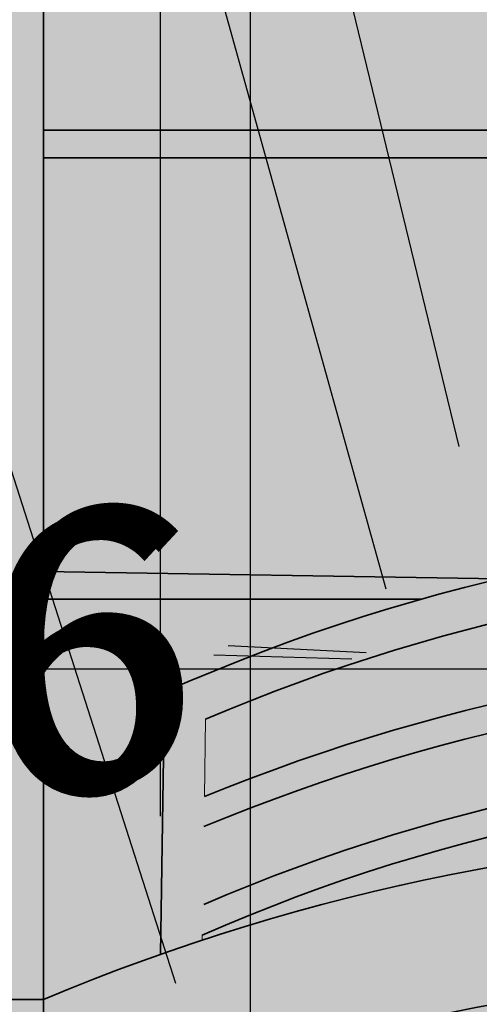
# Model space of a CAD drawing. Units: millimetres. Extents: x 130 to 1021, y 147 to 699.
# Tile 20 of 40: x 366 to 399, y 477 to 548. Entities that reach past the tile are written whole.
import ezdxf

# ---------------------------------------------------------------- set-up
doc = ezdxf.new("R2010")
doc.units = ezdxf.units.MM
doc.header["$MEASUREMENT"] = 0
for name, color, linetype, lineweight in [('A-ANNO-DIMS', 2, 'Continuous', 18), ('A-ELEV', 7, 'Continuous', 35), ('A-ELEV-PATT', 9, 'Continuous', 13), ('A-ELEV-RAIL', 6, 'Continuous', 18)]:
    doc.layers.add(name, color=color, linetype=linetype, lineweight=lineweight)
doc.styles.get("Standard").update_dxf_attribs({"font": 'arial.ttf'})
doc.dimstyles.get("Standard").update_dxf_attribs({"dimtxt": 20, "dimasz": 10, "dimexe": 10, "dimexo": 10, "dimgap": 5, "dimtad": 0, "dimtih": 1, "dimtoh": 1, "dimdec": 0, "dimzin": 0, "dimdsep": 46, "dimtxsty": 'Standard', "dimcen": 5, "dimadec": 0, "dimazin": 0, "dimtfac": 1, "dimtdec": 0, "dimtofl": 0, "dimtmove": 0, "dimatfit": 3, "dimfxl": 1, "dimtolj": 1, "dimtzin": 0, "dimarcsym": 0})

# ---------------------------------------------------------------- blocks, each defined once
blk = doc.blocks.new('*D11')
at = {"layer": 'A-ANNO-DIMS', "color": 0, "lineweight": -2, "transparency": 16777216}
for p, q in [((737.374, 648.699), (737.374, 149.739)), ((299.374, 566.947), (299.374, 149.739)), ((309.374, 159.739), (490.857, 159.739)), ((727.374, 159.739), (545.891, 159.739))]:
    blk.add_line(p, q, dxfattribs=at)
at = {"layer": 'A-ANNO-DIMS', "color": 0, "transparency": 16777216}
for points in [[(309.374, 161.406), (309.374, 158.073), (299.374, 159.739)], [(727.374, 161.406), (727.374, 158.073), (737.374, 159.739)]]:
    blk.add_solid(points, dxfattribs=at)
at = {"layer": 'Defpoints', "color": 0, "transparency": 16777216}
for p in [(737.374, 658.699), (299.374, 576.947), (737.374, 159.739)]:
    blk.add_point(p, dxfattribs=at)
at = {"layer": 'A-ANNO-DIMS', "color": 0, "transparency": 16777216, "insert": (518.374, 159.739), "char_height": 20, "attachment_point": 5}
blk.add_mtext('\\A1;438', dxfattribs=at)
blk = doc.blocks.new('*D12')
at = {"layer": 'A-ANNO-DIMS', "color": 0, "lineweight": -2, "transparency": 16777216}
for p, q in [((477.374, 661.947), (265.074, 661.947)), ((275.074, 651.947), (275.074, 438.205)), ((275.074, 194.039), (275.074, 407.782)), ((357.163, 184.039), (265.074, 184.039))]:
    blk.add_line(p, q, dxfattribs=at)
at = {"layer": 'A-ANNO-DIMS', "color": 0, "transparency": 16777216}
for points in [[(273.407, 651.947), (276.74, 651.947), (275.074, 661.947)], [(273.407, 194.039), (276.74, 194.039), (275.074, 184.039)]]:
    blk.add_solid(points, dxfattribs=at)
at = {"layer": 'Defpoints', "color": 0, "transparency": 16777216}
for p in [(275.074, 661.947), (487.374, 661.947), (367.163, 184.039)]:
    blk.add_point(p, dxfattribs=at)
at = {"layer": 'A-ANNO-DIMS', "color": 0, "transparency": 16777216, "insert": (275.074, 422.993), "char_height": 20, "attachment_point": 5}
blk.add_mtext('\\A1;477.9', dxfattribs=at)
blk = doc.blocks.new('*D15')
at = {"layer": 'A-ANNO-DIMS', "color": 0, "lineweight": -2, "transparency": 16777216}
for p, q in [((327.374, 579.884), (327.374, 696.247)), ((357.941, 411.947), (357.941, 696.247)), ((337.374, 686.247), (347.941, 686.247)), ((357.941, 686.247), (367.941, 686.247))]:
    blk.add_line(p, q, dxfattribs=at)
at = {"layer": 'A-ANNO-DIMS', "color": 0, "transparency": 16777216}
for points in [[(337.374, 687.914), (337.374, 684.581), (327.374, 686.247)], [(347.941, 687.914), (347.941, 684.581), (357.941, 686.247)]]:
    blk.add_solid(points, dxfattribs=at)
at = {"layer": 'Defpoints', "color": 0, "transparency": 16777216}
for p in [(357.941, 686.247), (327.374, 569.884), (357.941, 401.947)]:
    blk.add_point(p, dxfattribs=at)
at = {"layer": 'A-ANNO-DIMS', "color": 0, "transparency": 16777216, "insert": (406.679, 686.247), "char_height": 20, "attachment_point": 5}
blk.add_mtext('\\A1;30.57', dxfattribs=at)
blk = doc.blocks.new('*D16')
at = {"layer": 'A-ANNO-DIMS', "color": 0, "lineweight": -2, "transparency": 16777216}
for p, q in [((357.941, 411.947), (357.941, 696.247)), ((363.922, 579.884), (363.922, 696.247)), ((347.941, 686.247), (337.941, 686.247)), ((373.922, 686.247), (383.922, 686.247))]:
    blk.add_line(p, q, dxfattribs=at)
at = {"layer": 'A-ANNO-DIMS', "color": 0, "transparency": 16777216}
for points in [[(347.941, 687.914), (347.941, 684.581), (357.941, 686.247)], [(373.922, 687.914), (373.922, 684.581), (363.922, 686.247)]]:
    blk.add_solid(points, dxfattribs=at)
at = {"layer": 'Defpoints', "color": 0, "transparency": 16777216}
for p in [(363.922, 686.247), (363.922, 569.884), (357.941, 401.947)]:
    blk.add_point(p, dxfattribs=at)
at = {"layer": 'A-ANNO-DIMS', "color": 0, "transparency": 16777216, "insert": (420.737, 686.247), "char_height": 20, "attachment_point": 5}
blk.add_mtext('\\A1;5.981', dxfattribs=at)
blk = doc.blocks.new('*D17')
at = {"layer": 'A-ANNO-DIMS', "color": 0, "lineweight": -2, "transparency": 16777216}
for p, q in [((363.922, 579.884), (363.922, 696.247)), ((375.85, 490.216), (375.85, 696.247)), ((353.922, 686.247), (343.922, 686.247)), ((385.85, 686.247), (395.85, 686.247))]:
    blk.add_line(p, q, dxfattribs=at)
at = {"layer": 'A-ANNO-DIMS', "color": 0, "transparency": 16777216}
for points in [[(353.922, 687.914), (353.922, 684.581), (363.922, 686.247)], [(385.85, 687.914), (385.85, 684.581), (375.85, 686.247)]]:
    blk.add_solid(points, dxfattribs=at)
at = {"layer": 'Defpoints', "color": 0, "transparency": 16777216}
for p in [(375.85, 686.247), (363.922, 569.884), (375.85, 480.216)]:
    blk.add_point(p, dxfattribs=at)
at = {"layer": 'A-ANNO-DIMS', "color": 0, "transparency": 16777216, "insert": (441.444, 686.247), "char_height": 20, "attachment_point": 5}
blk.add_mtext('\\A1;11.928', dxfattribs=at)
blk = doc.blocks.new('*D18')
at = {"layer": 'A-ANNO-DIMS', "color": 0, "lineweight": -2, "transparency": 16777216}
for p, q in [((375.85, 490.216), (375.85, 696.247)), ((382.374, 388.947), (382.374, 696.247)), ((365.85, 686.247), (355.85, 686.247)), ((392.374, 686.247), (402.374, 686.247))]:
    blk.add_line(p, q, dxfattribs=at)
at = {"layer": 'A-ANNO-DIMS', "color": 0, "transparency": 16777216}
for points in [[(365.85, 687.914), (365.85, 684.581), (375.85, 686.247)], [(392.374, 687.914), (392.374, 684.581), (382.374, 686.247)]]:
    blk.add_solid(points, dxfattribs=at)
at = {"layer": 'Defpoints', "color": 0, "transparency": 16777216}
for p in [(382.374, 686.247), (375.85, 480.216), (382.374, 378.947)]:
    blk.add_point(p, dxfattribs=at)
at = {"layer": 'A-ANNO-DIMS', "color": 0, "transparency": 16777216, "insert": (441.132, 686.247), "char_height": 20, "attachment_point": 5}
blk.add_mtext('\\A1;6.524', dxfattribs=at)
blk = doc.blocks.new('*D19')
at = {"layer": 'A-ANNO-DIMS', "color": 0, "lineweight": -2, "transparency": 16777216}
for p, q in [((382.374, 388.947), (382.374, 696.247)), ((414.652, 510.881), (414.652, 696.247)), ((392.374, 686.247), (404.652, 686.247)), ((414.652, 686.247), (424.652, 686.247))]:
    blk.add_line(p, q, dxfattribs=at)
at = {"layer": 'A-ANNO-DIMS', "color": 0, "transparency": 16777216}
for points in [[(392.374, 687.914), (392.374, 684.581), (382.374, 686.247)], [(404.652, 687.914), (404.652, 684.581), (414.652, 686.247)]]:
    blk.add_solid(points, dxfattribs=at)
at = {"layer": 'Defpoints', "color": 0, "transparency": 16777216}
for p in [(414.652, 686.247), (414.652, 500.881), (382.374, 378.947)]:
    blk.add_point(p, dxfattribs=at)
at = {"layer": 'A-ANNO-DIMS', "color": 0, "transparency": 16777216, "insert": (463.411, 686.247), "char_height": 20, "attachment_point": 5}
blk.add_mtext('\\A1;32.28', dxfattribs=at)
blk = doc.blocks.new('*D20')
at = {"layer": 'A-ANNO-DIMS', "color": 0, "lineweight": -2, "transparency": 16777216}
for p, q in [((414.652, 510.881), (414.652, 696.247)), ((432.374, 388.947), (432.374, 696.247)), ((404.652, 686.247), (394.652, 686.247)), ((442.374, 686.247), (452.374, 686.247))]:
    blk.add_line(p, q, dxfattribs=at)
at = {"layer": 'A-ANNO-DIMS', "color": 0, "transparency": 16777216}
for points in [[(404.652, 687.914), (404.652, 684.581), (414.652, 686.247)], [(442.374, 687.914), (442.374, 684.581), (432.374, 686.247)]]:
    blk.add_solid(points, dxfattribs=at)
at = {"layer": 'Defpoints', "color": 0, "transparency": 16777216}
for p in [(432.374, 686.247), (414.652, 500.881), (432.374, 378.947)]:
    blk.add_point(p, dxfattribs=at)
at = {"layer": 'A-ANNO-DIMS', "color": 0, "transparency": 16777216, "insert": (490.075, 686.247), "char_height": 20, "attachment_point": 5}
blk.add_mtext('\\A1;17.72', dxfattribs=at)
blk = doc.blocks.new('*D43')
at = {"layer": 'A-ANNO-DIMS', "color": 0, "lineweight": -2, "transparency": 16777216}
for p, q in [((275.074, 510.881), (275.074, 520.881)), ((275.074, 520.881), (285.074, 520.881)), ((404.652, 500.881), (265.074, 500.881)), ((317.374, 480.95), (265.074, 480.95)), ((275.074, 470.95), (275.074, 460.95))]:
    blk.add_line(p, q, dxfattribs=at)
at = {"layer": 'A-ANNO-DIMS', "color": 0, "transparency": 16777216}
for points in [[(273.407, 510.881), (276.74, 510.881), (275.074, 500.881)], [(273.407, 470.95), (276.74, 470.95), (275.074, 480.95)]]:
    blk.add_solid(points, dxfattribs=at)
at = {"layer": 'Defpoints', "color": 0, "transparency": 16777216}
for p in [(275.074, 500.881), (414.652, 500.881), (327.374, 480.95)]:
    blk.add_point(p, dxfattribs=at)
at = {"layer": 'A-ANNO-DIMS', "color": 0, "transparency": 16777216, "insert": (322.877, 520.881), "char_height": 20, "attachment_point": 5}
blk.add_mtext('\\A1;19.93', dxfattribs=at)
blk = doc.blocks.new('*D44')
at = {"layer": 'A-ANNO-DIMS', "color": 0, "lineweight": -2, "transparency": 16777216}
for p, q in [((317.374, 569.884), (265.074, 569.884)), ((275.074, 559.884), (275.074, 550.594)), ((275.074, 510.881), (275.074, 520.171)), ((404.652, 500.881), (265.074, 500.881))]:
    blk.add_line(p, q, dxfattribs=at)
at = {"layer": 'A-ANNO-DIMS', "color": 0, "transparency": 16777216}
for points in [[(273.407, 559.884), (276.74, 559.884), (275.074, 569.884)], [(273.407, 510.881), (276.74, 510.881), (275.074, 500.881)]]:
    blk.add_solid(points, dxfattribs=at)
at = {"layer": 'Defpoints', "color": 0, "transparency": 16777216}
for p in [(275.074, 569.884), (327.374, 569.884), (414.652, 500.881)]:
    blk.add_point(p, dxfattribs=at)
at = {"layer": 'A-ANNO-DIMS', "color": 0, "transparency": 16777216, "insert": (275.074, 535.383), "char_height": 20, "attachment_point": 5}
blk.add_mtext('\\A1;69', dxfattribs=at)
blk = doc.blocks.new('*D62')
at = {"layer": 'A-ANNO-DIMS', "color": 0, "lineweight": -2, "transparency": 16777216}
for p, q in [((414.652, 495.881), (414.652, 505.881)), ((379.725, 501.926), (389.721, 501.627)), ((409.652, 500.881), (419.652, 500.881))]:
    blk.add_line(p, q, dxfattribs=at)
at = {"layer": 'A-ANNO-DIMS', "color": 0, "transparency": 16777216}
blk.add_solid([(389.771, 503.293), (389.671, 499.961), (399.716, 501.328)], dxfattribs=at)
at = {"layer": 'Defpoints', "color": 0, "transparency": 16777216}
for p in [(399.716, 501.328), (429.589, 500.434)]:
    blk.add_point(p, dxfattribs=at)
at = {"layer": 'A-ANNO-DIMS', "color": 0, "transparency": 16777216, "insert": (322.338, 501.926), "char_height": 20, "attachment_point": 5}
blk.add_mtext('\\A1;∅29.886', dxfattribs=at)
blk = doc.blocks.new('*D63')
at = {"layer": 'A-ANNO-DIMS', "color": 0, "lineweight": -2, "transparency": 16777216}
for p, q in [((414.652, 495.881), (414.652, 505.881)), ((380.753, 502.59), (390.74, 502.086)), ((409.652, 500.881), (419.652, 500.881))]:
    blk.add_line(p, q, dxfattribs=at)
at = {"layer": 'A-ANNO-DIMS', "color": 0, "transparency": 16777216}
blk.add_solid([(390.824, 503.751), (390.656, 500.422), (400.727, 501.583)], dxfattribs=at)
at = {"layer": 'Defpoints', "color": 0, "transparency": 16777216}
for p in [(400.727, 501.583), (428.578, 500.179)]:
    blk.add_point(p, dxfattribs=at)
at = {"layer": 'A-ANNO-DIMS', "color": 0, "transparency": 16777216, "insert": (323.365, 502.59), "char_height": 20, "attachment_point": 5}
blk.add_mtext('\\A1;∅27.886', dxfattribs=at)
blk = doc.blocks.new('*D66')
at = {"layer": 'A-ANNO-DIMS', "color": 0, "lineweight": -2, "transparency": 16777216}
for p, q in [((341.579, 557.194), (351.579, 557.194)), ((351.579, 557.194), (376.947, 478.135)), ((427.374, 315.978), (427.374, 325.978)), ((422.374, 320.978), (432.374, 320.978))]:
    blk.add_line(p, q, dxfattribs=at)
at = {"layer": 'A-ANNO-DIMS', "color": 0, "transparency": 16777216}
blk.add_solid([(378.534, 478.644), (375.36, 477.626), (380.002, 468.613)], dxfattribs=at)
at = {"layer": 'Defpoints', "color": 0, "transparency": 16777216}
for p in [(380.002, 468.613), (427.374, 320.978)]:
    blk.add_point(p, dxfattribs=at)
at = {"layer": 'A-ANNO-DIMS', "color": 0, "transparency": 16777216, "insert": (263.53, 557.194), "char_height": 20, "attachment_point": 5}
blk.add_mtext('\\A1;4X R155.05', dxfattribs=at)
blk = doc.blocks.new('*D68')
at = {"layer": 'A-ANNO-DIMS', "color": 0, "lineweight": -2, "transparency": 16777216}
for p, q in [((361.841, 579.756), (371.841, 579.756)), ((371.841, 579.756), (392.167, 506.693)), ((433.191, 354.23), (433.191, 364.23)), ((428.191, 359.23), (438.191, 359.23))]:
    blk.add_line(p, q, dxfattribs=at)
at = {"layer": 'A-ANNO-DIMS', "color": 0, "transparency": 16777216}
blk.add_solid([(393.773, 507.14), (390.561, 506.246), (394.847, 497.059)], dxfattribs=at)
at = {"layer": 'Defpoints', "color": 0, "transparency": 16777216}
for p in [(394.847, 497.059), (433.191, 359.23)]:
    blk.add_point(p, dxfattribs=at)
at = {"layer": 'A-ANNO-DIMS', "color": 0, "transparency": 16777216, "insert": (305.764, 579.756), "char_height": 20, "attachment_point": 5}
blk.add_mtext('\\A1;R143.06', dxfattribs=at)
blk = doc.blocks.new('*D70')
at = {"layer": 'A-ANNO-DIMS', "color": 0, "lineweight": -2, "transparency": 16777216}
for p, q in [((370.141, 588.4), (380.141, 588.4)), ((380.141, 588.4), (397.473, 517.008)), ((432.65, 367.109), (432.65, 377.109)), ((427.65, 372.109), (437.65, 372.109))]:
    blk.add_line(p, q, dxfattribs=at)
at = {"layer": 'A-ANNO-DIMS', "color": 0, "transparency": 16777216}
blk.add_solid([(399.093, 517.402), (395.854, 516.615), (399.832, 507.291)], dxfattribs=at)
at = {"layer": 'Defpoints', "color": 0, "transparency": 16777216}
for p in [(399.832, 507.291), (432.65, 372.109)]:
    blk.add_point(p, dxfattribs=at)
at = {"layer": 'A-ANNO-DIMS', "color": 0, "transparency": 16777216, "insert": (323.757, 588.4), "char_height": 20, "attachment_point": 5}
blk.add_mtext('\\A1;R139.1', dxfattribs=at)
blk = doc.blocks.new('*D73')
at = {"layer": 'A-ANNO-DIMS', "color": 0, "lineweight": -2, "transparency": 16777216}
for p, q in [((402.678, 571.448), (412.678, 571.448)), ((412.678, 571.448), (419.051, 502.166)), ((432.115, 355.142), (432.115, 365.142)), ((427.115, 360.142), (437.115, 360.142))]:
    blk.add_line(p, q, dxfattribs=at)
at = {"layer": 'A-ANNO-DIMS', "color": 0, "transparency": 16777216}
blk.add_solid([(420.711, 502.319), (417.391, 502.014), (419.967, 492.208)], dxfattribs=at)
at = {"layer": 'Defpoints', "color": 0, "transparency": 16777216}
for p in [(419.967, 492.208), (432.115, 360.142)]:
    blk.add_point(p, dxfattribs=at)
at = {"layer": 'A-ANNO-DIMS', "color": 0, "transparency": 16777216, "insert": (346.696, 571.448), "char_height": 20, "attachment_point": 5}
blk.add_mtext('\\A1;R132.62', dxfattribs=at)

msp = doc.modelspace()

# ---------------------------------------------------------------- hatches: boundary and pattern name
at = {"layer": 'A-ELEV-PATT'}
h = msp.add_hatch(color=256, dxfattribs=at)
h.dxf.hatch_style = 1
h.paths.add_polyline_path([(737.3738, 658.6988, 0.0135961), (632.4019, 661.9473), (607.3738, 661.9473), (487.3738, 661.9473), (487.3738, 649.9473), (607.3738, 649.9473), (632.3794, 649.9473, -0.0136841), (737.3738, 646.6784)])
h.paths.add_polyline_path([(732.3738, 643.9599, 0.0130529), (632.3738, 646.9473), (607.3738, 646.9473), (487.3738, 646.9473), (487.3738, 596.9473), (632.3738, 596.9473, -0.0130529), (732.3738, 593.9599)])
h.paths.add_polyline_path([(737.3738, 593.6732, 0.0137063), (632.3738, 596.9473), (487.3738, 596.9473), (487.3738, 586.9473), (632.355, 586.9473, -0.0137808), (737.3738, 583.6559)])
h.paths.add_polyline_path([(447.3738, 646.9473), (307.3738, 646.9473), (302.3738, 646.9473), (302.3738, 634.9473), (447.3738, 634.9473)])
h.paths.add_polyline_path([(447.3738, 631.9473), (307.3738, 631.9473), (307.3738, 586.9473), (447.3738, 586.9473)])
h.paths.add_polyline_path([(447.3738, 586.9473), (307.3738, 586.9473), (302.3738, 586.9473), (302.3738, 576.9473), (447.3738, 576.9473)])
h.paths.add_polyline_path([(447.3738, 573.9473), (367.3738, 573.9473), (367.3738, 539.9473), (447.3738, 539.9473)])
h.paths.add_polyline_path([(447.3738, 537.9473), (367.3738, 537.9473), (367.3738, 507.9473), (400.392, 507.4253, -0.001728), (401.3281, 507.6451, -0.5220025), (425.6117, 511.0391, -0.0391849), (447.3738, 510.4359), (447.3738, 510.7883)])
h.paths.add_polyline_path([(394.7238, 505.9473), (367.3738, 505.9473), (367.3738, 476.9473, -0.0146512), (375.8501, 480.2159), (376.1506, 499.2266, -0.0355419)])
h.paths.add_polyline_path([(632.3738, 583.9473), (552.3738, 583.9473), (552.3738, 550.9473), (632.3738, 550.9473)])
h.paths.add_polyline_path([(632.3738, 548.9473), (552.3738, 548.9473), (552.3738, 515.9473), (632.3738, 515.9473)])
h.paths.add_polyline_path([(632.3738, 513.9473), (552.3738, 513.9473), (552.3738, 476.9473), (632.3738, 476.9473)])
h.paths.add_polyline_path([(737.3738, 473.6903, 0.0136326), (632.3926, 476.9473), (552.3738, 476.9473), (487.3738, 476.9473), (487.3738, 466.9473), (632.3738, 466.9473, -0.0137063), (737.3738, 463.6732)])
h.paths.add_polyline_path([(732.3738, 460.9552, 0.0130741), (632.3681, 463.9473), (487.3738, 463.9473), (487.3738, 407.735, -0.0032286), (489.3544, 406.9473), (632.3926, 406.9473, -0.0129826), (732.3738, 403.9755)])
h.paths.add_polyline_path([(487.3738, 463.9473, 0.20133), (367.3738, 463.9473), (367.3738, 407.735, -0.1882031), (487.3738, 407.735)])
h.paths.add_polyline_path([(367.3738, 476.9473), (367.3738, 466.9473, -0.2013309), (487.3738, 466.9473), (487.3738, 476.9473, 0.20133)])
h.paths.add_polyline_path([(367.3738, 463.9473), (307.3738, 463.9473), (307.3738, 401.9473), (357.9413, 401.9473), (367.3738, 407.735)])
h.paths.add_polyline_path([(367.3738, 476.9473), (302.3738, 476.9473), (302.3738, 466.9473), (367.3738, 466.9473)])
h.paths.add_polyline_path([(632.8184, 366.9453), (552.3738, 366.9453), (552.3738, 393.9473), (632.8184, 393.9473)])
h.paths.add_polyline_path([(632.8184, 357.2114), (632.8184, 363.9453), (552.3738, 363.9453), (552.3738, 357.2114), (552.3738, 336.9453), (632.8184, 336.9453)])
h.paths.add_polyline_path([(632.8184, 333.9453), (552.3738, 333.9453), (552.3738, 306.9453), (632.8184, 306.9453)])
h.paths.add_polyline_path([(632.8184, 303.9453), (552.3738, 303.9453), (552.3738, 273.9473), (632.355, 273.9473, 0.0000608), (632.8184, 273.9491)])
h.paths.add_polyline_path([(737.3738, 403.6903, 0.0136326), (632.3926, 406.9473), (489.3544, 406.9473, 0.1915481), (367.3738, 407.735), (367.3738, 396.9473, -0.2013309), (487.3738, 396.9473), (632.3738, 396.9473, -0.0137063), (737.3738, 393.6732)])
h.paths.add_polyline_path([(357.9413, 401.9473), (307.3738, 401.9473), (307.3738, 391.9473), (357.9413, 391.9473)])
h.paths.add_polyline_path([(357.9413, 357.2114), (357.9413, 388.9473), (307.3738, 388.9473), (307.3738, 357.2114), (307.3738, 273.9473), (357.9413, 273.9473)])
h.paths.add_polyline_path([(732.3738, 263.93, -0.0130317), (632.3794, 260.9473), (466.7667, 260.9473), (466.7667, 240.9473), (469.8406, 236.978), (469.8406, 221.978), (472.9145, 218.0087), (472.9145, 213.9473), (607.3738, 213.9473), (732.3738, 213.9473)])
h.paths.add_polyline_path([(732.3738, 290.889), (722.479, 290.889), (722.479, 301.889), (732.3738, 301.889), (732.3738, 305.889), (722.479, 305.889), (722.479, 316.889), (732.3738, 316.889), (732.3738, 320.889), (722.479, 320.889), (722.479, 331.889), (732.3738, 331.889), (732.3738, 335.889), (722.479, 335.889), (722.479, 346.889), (732.3738, 346.889), (732.3738, 350.889), (722.479, 350.889), (722.479, 361.889), (732.3738, 361.889), (732.3738, 365.889), (722.479, 365.889), (722.479, 376.889), (732.3738, 376.889), (732.3738, 380.889), (722.479, 380.889), (722.479, 391.4848, 0.0005233), (718.479, 391.6843), (718.479, 380.889), (707.479, 380.889), (707.479, 392.1896, 0.0005231), (703.479, 392.3576), (703.479, 380.889), (692.479, 380.889), (692.479, 392.7765, 0.0005229), (688.479, 392.9131), (688.479, 380.889), (677.479, 380.889), (677.479, 393.2456, 0.0005228), (673.479, 393.3508), (673.479, 380.889), (662.479, 380.889), (662.479, 393.597, 0.0005227), (658.479, 393.6709), (658.479, 380.889), (647.479, 380.889), (647.479, 393.8308, 0.0005226), (643.479, 393.8732), (643.479, 380.889), (632.8184, 380.889), (632.8184, 376.889), (643.479, 376.889), (643.479, 365.889), (632.8184, 365.889), (632.8184, 361.889), (643.479, 361.889), (643.479, 350.889), (632.8184, 350.889), (632.8184, 346.889), (643.479, 346.889), (643.479, 335.889), (632.8184, 335.889), (632.8184, 331.889), (643.479, 331.889), (643.479, 320.889), (632.8184, 320.889), (632.8184, 316.889), (643.479, 316.889), (643.479, 305.889), (632.8184, 305.889), (632.8184, 301.889), (643.479, 301.889), (643.479, 290.889), (632.8184, 290.889), (632.8184, 286.889), (643.479, 286.889), (643.479, 274.0217, 0.0005246), (647.479, 274.0643), (647.479, 286.889), (658.479, 286.889), (658.479, 274.2248, 0.0005246), (662.479, 274.2989), (662.479, 286.889), (673.479, 286.889), (673.479, 274.546, 0.0005247), (677.479, 274.6516), (677.479, 286.889), (688.479, 286.889), (688.479, 274.9853, 0.0005248), (692.479, 275.1224), (692.479, 286.889), (703.479, 286.889), (703.479, 275.5429, 0.000525), (707.479, 275.7115), (707.479, 286.889), (718.479, 286.889), (718.479, 276.2187, 0.0005252), (722.479, 276.4189), (722.479, 286.889), (732.3738, 286.889)])
h.paths.add_polyline_path([(718.479, 290.889), (707.479, 290.889), (707.479, 301.889), (718.479, 301.889)], flags=16)
h.paths.add_polyline_path([(703.479, 290.889), (692.479, 290.889), (692.479, 301.889), (703.479, 301.889)], flags=16)
h.paths.add_polyline_path([(718.479, 305.889), (707.479, 305.889), (707.479, 316.889), (718.479, 316.889)], flags=16)
h.paths.add_polyline_path([(703.479, 305.889), (692.479, 305.889), (692.479, 316.889), (703.479, 316.889)], flags=16)
h.paths.add_polyline_path([(688.479, 290.889), (677.479, 290.889), (677.479, 301.889), (688.479, 301.889)], flags=16)
h.paths.add_polyline_path([(718.479, 320.889), (707.479, 320.889), (707.479, 331.889), (718.479, 331.889)], flags=16)
h.paths.add_polyline_path([(688.479, 305.889), (677.479, 305.889), (677.479, 316.889), (688.479, 316.889)], flags=16)
h.paths.add_polyline_path([(703.479, 320.889), (692.479, 320.889), (692.479, 331.889), (703.479, 331.889)], flags=16)
h.paths.add_polyline_path([(688.479, 320.889), (677.479, 320.889), (677.479, 331.889), (688.479, 331.889)], flags=16)
h.paths.add_polyline_path([(673.479, 290.889), (662.479, 290.889), (662.479, 301.889), (673.479, 301.889)], flags=16)
h.paths.add_polyline_path([(718.479, 335.889), (707.479, 335.889), (707.479, 346.889), (718.479, 346.889)], flags=16)
h.paths.add_polyline_path([(673.479, 305.889), (662.479, 305.889), (662.479, 316.889), (673.479, 316.889)], flags=16)
h.paths.add_polyline_path([(703.479, 335.889), (692.479, 335.889), (692.479, 346.889), (703.479, 346.889)], flags=16)
h.paths.add_polyline_path([(673.479, 320.889), (662.479, 320.889), (662.479, 331.889), (673.479, 331.889)], flags=16)
h.paths.add_polyline_path([(688.479, 335.889), (677.479, 335.889), (677.479, 346.889), (688.479, 346.889)], flags=16)
h.paths.add_polyline_path([(658.479, 290.889), (647.479, 290.889), (647.479, 301.889), (658.479, 301.889)], flags=16)
h.paths.add_polyline_path([(718.479, 350.889), (707.479, 350.889), (707.479, 361.889), (718.479, 361.889)], flags=16)
h.paths.add_polyline_path([(658.479, 305.889), (647.479, 305.889), (647.479, 316.889), (658.479, 316.889)], flags=16)
h.paths.add_polyline_path([(703.479, 350.889), (692.479, 350.889), (692.479, 361.889), (703.479, 361.889)], flags=16)
h.paths.add_polyline_path([(673.479, 335.889), (662.479, 335.889), (662.479, 346.889), (673.479, 346.889)], flags=16)
h.paths.add_polyline_path([(658.479, 320.889), (647.479, 320.889), (647.479, 331.889), (658.479, 331.889)], flags=16)
h.paths.add_polyline_path([(688.479, 350.889), (677.479, 350.889), (677.479, 361.889), (688.479, 361.889)], flags=16)
h.paths.add_polyline_path([(718.479, 365.889), (707.479, 365.889), (707.479, 376.889), (718.479, 376.889)], flags=16)
h.paths.add_polyline_path([(658.479, 335.889), (647.479, 335.889), (647.479, 346.889), (658.479, 346.889)], flags=16)
h.paths.add_polyline_path([(673.479, 350.889), (662.479, 350.889), (662.479, 361.889), (673.479, 361.889)], flags=16)
h.paths.add_polyline_path([(703.479, 365.889), (692.479, 365.889), (692.479, 376.889), (703.479, 376.889)], flags=16)
h.paths.add_polyline_path([(688.479, 365.889), (677.479, 365.889), (677.479, 376.889), (688.479, 376.889)], flags=16)
h.paths.add_polyline_path([(658.479, 350.889), (647.479, 350.889), (647.479, 361.889), (658.479, 361.889)], flags=16)
h.paths.add_polyline_path([(673.479, 365.889), (662.479, 365.889), (662.479, 376.889), (673.479, 376.889)], flags=16)
h.paths.add_polyline_path([(658.479, 365.889), (647.479, 365.889), (647.479, 376.889), (658.479, 376.889)], flags=16)
h.paths.add_polyline_path([(732.3738, 503.9786), (722.3392, 503.9786), (722.3392, 514.9786), (732.3738, 514.9786), (732.3738, 518.9786), (722.3392, 518.9786), (722.3392, 529.9786), (732.3738, 529.9786), (732.3738, 533.9786), (722.3392, 533.9786), (722.3392, 544.9786), (732.3738, 544.9786), (732.3738, 546.9473), (732.3738, 548.9786), (722.3392, 548.9786), (722.3392, 559.9786), (732.3738, 559.9786), (732.3738, 563.9786), (722.3392, 563.9786), (722.3392, 574.9786), (732.3738, 574.9786), (732.3738, 578.9786), (722.3392, 578.9786), (722.3392, 581.4789, 0.000526), (718.3392, 581.6791), (718.3392, 578.9786), (707.3392, 578.9786), (707.3392, 582.1863, 0.0005258), (703.3392, 582.355), (703.3392, 578.9786), (692.3392, 578.9786), (692.3392, 582.7752, 0.0005257), (688.3392, 582.9123), (688.3392, 578.9786), (677.3392, 578.9786), (677.3392, 583.2457, 0.0005255), (673.3392, 583.3512), (673.3392, 578.9786), (662.3392, 578.9786), (662.3392, 583.5978, 0.0005254), (658.3392, 583.6718), (658.3392, 578.9786), (647.3392, 578.9786), (647.3392, 583.8317, 0.0005254), (643.3392, 583.8741), (643.3392, 578.9786), (632.3738, 578.9786), (632.3738, 574.9786), (643.3392, 574.9786), (643.3392, 563.9786), (632.3738, 563.9786), (632.3738, 559.9786), (643.3392, 559.9786), (643.3392, 548.9786), (632.3738, 548.9786), (632.3738, 544.9786), (643.3392, 544.9786), (643.3392, 533.9786), (632.3738, 533.9786), (632.3738, 529.9786), (643.3392, 529.9786), (643.3392, 518.9786), (632.3738, 518.9786), (632.3738, 515.9473), (632.3738, 514.9786), (643.3392, 514.9786), (643.3392, 503.9786), (632.3738, 503.9786), (632.3738, 499.9786), (643.3392, 499.9786), (643.3392, 488.9786), (632.3738, 488.9786), (632.3738, 484.9786), (643.3392, 484.9786), (643.3392, 476.8751, -0.0005191), (647.3392, 476.8332), (647.3392, 484.9786), (658.3392, 484.9786), (658.3392, 476.6752, -0.0005192), (662.3392, 476.6022), (662.3392, 484.9786), (673.3392, 484.9786), (673.3392, 476.3585, -0.0005193), (677.3392, 476.2543), (677.3392, 484.9786), (688.3392, 484.9786), (688.3392, 475.9248, -0.0005194), (692.3392, 475.7894), (692.3392, 484.9786), (703.3392, 484.9786), (703.3392, 475.3741, -0.0005195), (707.3392, 475.2075), (707.3392, 484.9786), (718.3392, 484.9786), (718.3392, 474.7064, -0.0005197), (722.3392, 474.5086), (722.3392, 484.9786), (732.3738, 484.9786), (732.3738, 488.9786), (722.3392, 488.9786), (722.3392, 499.9786), (732.3738, 499.9786)])
h.paths.add_polyline_path([(718.3392, 503.9786), (707.3392, 503.9786), (707.3392, 514.9786), (718.3392, 514.9786)], flags=16)
h.paths.add_polyline_path([(718.3392, 499.9786), (718.3392, 488.9786), (707.3392, 488.9786), (707.3392, 499.9786)], flags=16)
h.paths.add_polyline_path([(718.3392, 518.9786), (707.3392, 518.9786), (707.3392, 529.9786), (718.3392, 529.9786)], flags=16)
h.paths.add_polyline_path([(703.3392, 503.9786), (692.3392, 503.9786), (692.3392, 514.9786), (703.3392, 514.9786)], flags=16)
h.paths.add_polyline_path([(703.3392, 499.9786), (703.3392, 488.9786), (692.3392, 488.9786), (692.3392, 499.9786)], flags=16)
h.paths.add_polyline_path([(703.3392, 518.9786), (692.3392, 518.9786), (692.3392, 529.9786), (703.3392, 529.9786)], flags=16)
h.paths.add_polyline_path([(718.3392, 533.9786), (707.3392, 533.9786), (707.3392, 544.9786), (718.3392, 544.9786)], flags=16)
h.paths.add_polyline_path([(688.3392, 503.9786), (677.3392, 503.9786), (677.3392, 514.9786), (688.3392, 514.9786)], flags=16)
h.paths.add_polyline_path([(688.3392, 499.9786), (688.3392, 488.9786), (677.3392, 488.9786), (677.3392, 499.9786)], flags=16)
h.paths.add_polyline_path([(703.3392, 533.9786), (692.3392, 533.9786), (692.3392, 544.9786), (703.3392, 544.9786)], flags=16)
h.paths.add_polyline_path([(688.3392, 518.9786), (677.3392, 518.9786), (677.3392, 529.9786), (688.3392, 529.9786)], flags=16)
h.paths.add_polyline_path([(688.3392, 533.9786), (677.3392, 533.9786), (677.3392, 544.9786), (688.3392, 544.9786)], flags=16)
h.paths.add_polyline_path([(718.3392, 548.9786), (707.3392, 548.9786), (707.3392, 559.9786), (718.3392, 559.9786)], flags=16)
h.paths.add_polyline_path([(673.3392, 503.9786), (662.3392, 503.9786), (662.3392, 514.9786), (673.3392, 514.9786)], flags=16)
h.paths.add_polyline_path([(673.3392, 499.9786), (673.3392, 488.9786), (662.3392, 488.9786), (662.3392, 499.9786)], flags=16)
h.paths.add_polyline_path([(703.3392, 548.9786), (692.3392, 548.9786), (692.3392, 559.9786), (703.3392, 559.9786)], flags=16)
h.paths.add_polyline_path([(673.3392, 518.9786), (662.3392, 518.9786), (662.3392, 529.9786), (673.3392, 529.9786)], flags=16)
h.paths.add_polyline_path([(688.3392, 548.9786), (677.3392, 548.9786), (677.3392, 559.9786), (688.3392, 559.9786)], flags=16)
h.paths.add_polyline_path([(673.3392, 533.9786), (662.3392, 533.9786), (662.3392, 544.9786), (673.3392, 544.9786)], flags=16)
h.paths.add_polyline_path([(718.3392, 563.9786), (707.3392, 563.9786), (707.3392, 574.9786), (718.3392, 574.9786)], flags=16)
h.paths.add_polyline_path([(658.3392, 503.9786), (647.3392, 503.9786), (647.3392, 514.9786), (658.3392, 514.9786)], flags=16)
h.paths.add_polyline_path([(658.3392, 499.9786), (658.3392, 488.9786), (647.3392, 488.9786), (647.3392, 499.9786)], flags=16)
h.paths.add_polyline_path([(703.3392, 563.9786), (692.3392, 563.9786), (692.3392, 574.9786), (703.3392, 574.9786)], flags=16)
h.paths.add_polyline_path([(658.3392, 518.9786), (647.3392, 518.9786), (647.3392, 529.9786), (658.3392, 529.9786)], flags=16)
h.paths.add_polyline_path([(673.3392, 548.9786), (662.3392, 548.9786), (662.3392, 559.9786), (673.3392, 559.9786)], flags=16)
h.paths.add_polyline_path([(688.3392, 563.9786), (677.3392, 563.9786), (677.3392, 574.9786), (688.3392, 574.9786)], flags=16)
h.paths.add_polyline_path([(658.3392, 533.9786), (647.3392, 533.9786), (647.3392, 544.9786), (658.3392, 544.9786)], flags=16)
h.paths.add_polyline_path([(673.3392, 563.9786), (662.3392, 563.9786), (662.3392, 574.9786), (673.3392, 574.9786)], flags=16)
h.paths.add_polyline_path([(658.3392, 548.9786), (647.3392, 548.9786), (647.3392, 559.9786), (658.3392, 559.9786)], flags=16)
h.paths.add_polyline_path([(658.3392, 563.9786), (647.3392, 563.9786), (647.3392, 574.9786), (658.3392, 574.9786)], flags=16)
h = msp.add_hatch(color=256, dxfattribs=at)
h.dxf.hatch_style = 1
h.paths.add_polyline_path([(447.3738, 576.9473), (302.3738, 576.9473), (302.3738, 573.9473), (447.3738, 573.9473)])
h.paths.add_polyline_path([(487.3738, 583.9473), (487.3738, 586.9473), (447.3738, 576.9473), (447.3738, 573.9473)])
h.paths.add_polyline_path([(632.355, 586.9473), (487.3738, 586.9473), (487.3738, 583.9473), (632.3738, 583.9473), (632.3738, 583.9472, -0.0138), (737.3738, 580.6507), (737.3738, 583.6559, 0.0137808)])
h.paths.add_polyline_path([(367.3738, 466.9473), (302.3738, 466.9473), (302.3738, 463.9473), (367.3738, 463.9473)])
h.paths.add_polyline_path([(487.3738, 463.9473), (487.3738, 466.9473, 0.2013309), (367.3738, 466.9473), (367.3738, 463.9473, -0.20133)])
h.paths.add_polyline_path([(632.3738, 466.9473), (487.3738, 466.9473), (487.3738, 463.9473), (632.3681, 463.9473, -0.0137285), (737.3738, 460.6681), (737.3738, 463.6732, 0.0137063)])
h.paths.add_polyline_path([(632.3738, 396.9473), (487.3738, 396.9473, 0.2013309), (367.3738, 396.9473), (367.3738, 393.9473, -0.2023717), (486.7667, 393.9473), (632.3681, 393.9473, -0.0137285), (737.3738, 390.6681), (737.3738, 393.6732, 0.0137063)])
h.paths.add_polyline_path([(357.9413, 391.9473), (307.3738, 391.9473), (307.3738, 388.9473), (357.9413, 388.9473)])
h.paths.add_polyline_path([(367.3738, 393.9473), (367.3738, 396.9473), (357.9413, 391.924), (357.9413, 388.9473), (358.058, 388.9473)])
h.paths.add_polyline_path([(737.3738, 264.2162), (737.3738, 267.2214, -0.0137063), (632.3738, 263.9473), (463.7667, 263.9473), (466.7667, 260.9473), (632.3794, 260.9473, 0.0136841)])
h.paths.add_polyline_path([(463.7667, 263.9473), (447.3738, 263.9473), (450.3738, 260.9473), (466.7667, 260.9473)])
h.paths.add_polyline_path([(447.3738, 263.9473), (432.3738, 263.9473), (432.3738, 260.9473), (450.3738, 260.9473)])
h.paths.add_polyline_path([(382.3738, 263.9473), (357.9413, 263.9473), (357.9413, 260.9473), (382.3738, 260.9473)])
h.paths.add_polyline_path([(357.9413, 263.9473), (307.3738, 263.9473), (307.3738, 260.9473), (357.9413, 260.9473)])
msp.add_hatch(color=256, dxfattribs=at).paths.add_polyline_path([(327.3738, 573.9473), (327.3738, 569.884), (363.922, 569.884), (363.922, 480.95), (327.3738, 480.95), (327.3738, 476.9473), (367.3738, 476.9473), (367.3738, 573.9473)])
h = msp.add_hatch(color=256, dxfattribs=at)
h.dxf.hatch_style = 1
h.paths.add_polyline_path([(447.3738, 537.9473), (447.3738, 539.9473), (367.3738, 539.9473), (367.3738, 537.9473)])
h.paths.add_polyline_path([(394.7238, 505.9473, -0.0105284), (400.392, 507.4253), (367.3738, 507.9473), (367.3738, 505.9473)])
h.paths.add_polyline_path([(547.7773, 546.9473), (547.7773, 548.9473), (502.3738, 548.9473), (502.3738, 546.9473)])
h.paths.add_polyline_path([(632.3738, 548.9473), (632.3738, 550.9473), (552.3738, 550.9473), (552.3738, 548.9473)])
h.paths.add_polyline_path([(632.3738, 513.9473), (632.3738, 515.9473), (552.3738, 515.9473), (552.3738, 513.9473)])
h.paths.add_polyline_path([(544.6354, 360.9453), (544.6354, 363.9453), (486.7667, 363.9454), (486.7667, 360.9454)])
h.paths.add_polyline_path([(632.8184, 363.9453), (632.8184, 366.9453), (552.3738, 366.9453), (552.3738, 363.9453)])
h.paths.add_polyline_path([(632.8184, 333.9453), (632.8184, 336.9453), (552.3738, 336.9453), (552.3738, 333.9453)])
h.paths.add_polyline_path([(552.3738, 306.9453), (552.3738, 303.9453), (632.8184, 303.9453), (632.8184, 306.9453)])
h = msp.add_hatch(color=256, dxfattribs=at)
h.paths.add_polyline_path([(375.8501, 480.2159, -0.0051389), (378.8667, 481.244), (378.8725, 481.6093, -0.2220519), (491.1023, 478.9257), (491.1023, 476.9473), (494.1023, 476.9473), (494.1023, 496.908, 0.2225165), (376.1506, 499.2266)])
h.paths.add_polyline_path([(379.1197, 497.2486, -0.2152592), (491.1023, 495.0271), (491.1023, 490.0474, 0.2040153), (379.0311, 491.6449)], flags=16)
h.paths.add_polyline_path([(491.1023, 487.8572), (491.1023, 481.1546, 0.1695534), (402.9637, 491.5717, -0.0927216), (400.3891, 496.4261, -0.1659296)], flags=16)
h = msp.add_hatch(color=256, dxfattribs=at)
h.paths.add_polyline_path([(399.9219, 498.3708, -0.0996756), (400.0983, 504.2673, 0.0406995), (379.1197, 497.2486), (379.0311, 491.6449, -0.0384084)])
h.paths.add_polyline_path([(402.9637, 491.5717, -0.0927216), (400.3891, 496.4261, 0.0399321), (378.9967, 489.4672), (378.9072, 483.8048, -0.0470483)])
h.paths.add_polyline_path([(404.5509, 489.8698, 0.0509798), (378.8725, 481.6093), (378.8667, 481.244, -0.0474823), (407.5193, 487.7506, -0.061248)])
h.paths.add_polyline_path([(447.3738, 491.8851, 0.0382282), (427.1388, 492.6724, -0.0850627), (423.6933, 488.9834, -0.0382916), (447.3738, 487.7318)])
h.paths.add_polyline_path([(447.3738, 499.578, 0.0315856), (429.5819, 500.2467, -0.0960946), (428.2619, 494.7107, -0.0355683), (447.3738, 493.8983)])
h.paths.add_polyline_path([(447.3738, 507.4186, 0.0361693), (427.7205, 508.128, -0.1040877), (429.5329, 502.2461, -0.0312283), (447.3738, 501.588)])

# ---------------------------------------------------------------- linework, layer by layer
at = {"layer": 'A-ELEV'}
for p, q in [((367.3738, 573.9473), (367.3738, 357.2114)), ((367.3738, 541.9473), (367.3738, 539.9473)), ((367.3738, 539.9473), (447.3738, 539.9473)), ((367.3738, 537.9473), (447.3738, 537.9473)), ((367.3738, 509.9473), (367.3738, 507.9473)), ((367.3738, 507.9473), (400.392, 507.4253)), ((367.3738, 505.9473), (394.7238, 505.9473)), ((376.1506, 499.2266), (375.8501, 480.2159)), ((367.3738, 476.9473), (302.3738, 476.9473))]:
    msp.add_line(p, q, dxfattribs=at)
for centre, radius, start, end in [((432.6505, 372.1087), 139.1086, 63.78413, 113.963624), ((432.6505, 372.1087), 136.1086, 64.567343, 113.15965), ((433.1906, 359.2304), 143.0624, 66.12141, 112.245303), ((433.1906, 359.2304), 141.0624, 65.761287, 112.593106), ((432.115, 360.1423), 134.6235, 64.013142, 113.246941), ((432.115, 360.1423), 132.6235, 63.591208, 113.669232), ((427.3738, 333.9781), 155.049, 67.23363, 112.76637), ((427.3738, 323.9788), 155.0484, 67.233534, 112.766466)]:
    msp.add_arc(centre, radius, start, end, dxfattribs=at)
at = {"layer": 'A-ELEV-RAIL'}
for p, q in [((379.1197, 497.2486), (379.0311, 491.6449)), ((378.8725, 481.6093), (378.8667, 481.244))]:
    msp.add_line(p, q, dxfattribs=at)

# ---------------------------------------------------------------- dimensions: what is measured, and where the dimension line sits
at = {"layer": 'A-ANNO-DIMS'}
for base, p1, p2, override, picture, middle in [((357.9413, 686.2473), (327.3738, 569.884), (357.9413, 401.9473), {"dimdec": 2, "dimlfac": 1, "dimrnd": 0, "dimzin": 0, "dimdsep": 46, "dimlunit": 2}, '*D15', (406.6794, 686.2473)), ((363.922, 686.2473), (357.9413, 401.9473), (363.922, 569.884), {"dimdec": 3, "dimlfac": 1, "dimrnd": 0, "dimzin": 0, "dimdsep": 46, "dimlunit": 2}, '*D16', (420.7365, 686.2473)), ((375.8501, 686.2473), (363.922, 569.884), (375.8501, 480.2159), {"dimdec": 3, "dimlfac": 1, "dimrnd": 0, "dimzin": 0, "dimdsep": 46, "dimlunit": 2}, '*D17', (441.4435, 686.2473)), ((382.3738, 686.2473), (375.8501, 480.2159), (382.3738, 378.9473), {"dimdec": 3, "dimlfac": 1, "dimrnd": 0, "dimzin": 0, "dimdsep": 46, "dimlunit": 2}, '*D18', (441.1323, 686.2473)), ((414.6525, 686.2473), (382.3738, 378.9473), (414.6525, 500.8811), {"dimdec": 2, "dimlfac": 1, "dimrnd": 0, "dimzin": 0, "dimdsep": 46, "dimlunit": 2}, '*D19', (463.411, 686.2473)), ((432.3738, 686.2473), (414.6525, 500.8811), (432.3738, 378.9473), {"dimdec": 2, "dimlfac": 1, "dimrnd": 0, "dimzin": 0, "dimdsep": 46, "dimlunit": 2}, '*D20', (490.075, 686.2473)), ((737.3738, 159.7395), (299.3738, 576.9473), (737.3738, 658.6988), {"dimdec": 0, "dimlfac": 1, "dimrnd": 0, "dimzin": 0, "dimdsep": 46, "dimlunit": 2}, '*D11', (518.3738, 159.7395))]:
    dim = msp.add_linear_dim(base=base, p1=p1, p2=p2, dimstyle='Standard', override=override, dxfattribs=at)
    dim.commit()
    dim.dimension.update_dxf_attribs({"geometry": picture, "text_midpoint": middle})
for base, p1, p2, override, picture, middle in [((275.0738, 661.9473), (367.163, 184.0395), (487.3738, 661.9473), {"dimdec": 1, "dimlfac": 1, "dimrnd": 0, "dimzin": 0, "dimdsep": 46, "dimlunit": 2}, '*D12', (275.0738, 422.9934)), ((275.0738, 569.884), (414.6525, 500.8811), (327.3738, 569.884), {"dimdec": 0, "dimlfac": 1, "dimrnd": 0, "dimzin": 0, "dimdsep": 46, "dimlunit": 2}, '*D44', (275.0738, 535.3826)), ((275.0738, 500.8811), (327.3738, 480.95), (414.6525, 500.8811), {"dimdec": 2, "dimlfac": 1, "dimrnd": 0, "dimzin": 0, "dimdsep": 46, "dimlunit": 2}, '*D43', (322.8773, 520.8811))]:
    dim = msp.add_linear_dim(base=base, p1=p1, p2=p2, angle=90, dimstyle='Standard', override=override, dxfattribs=at)
    dim.commit()
    dim.dimension.update_dxf_attribs({"geometry": picture, "text_midpoint": middle})
for center, mpoint, override, picture, middle in [((432.6505, 372.1087), (399.8323, 507.2907), {"dimdec": 1, "dimlfac": 1, "dimrnd": 0, "dimzin": 0, "dimdsep": 46, "dimlunit": 2}, '*D70', (323.7567, 588.3999)), ((433.1906, 359.2304), (394.8473, 497.0587), {"dimdec": 2, "dimlfac": 1, "dimrnd": 0, "dimzin": 0, "dimdsep": 46, "dimlunit": 2}, '*D68', (305.7636, 579.7557)), ((432.115, 360.1423), (419.967, 492.2083), {"dimdec": 2, "dimlfac": 1, "dimrnd": 0, "dimzin": 0, "dimdsep": 46, "dimlunit": 2}, '*D73', (346.696, 571.4479))]:
    dim = msp.add_radius_dim(center=center, mpoint=mpoint, dimstyle='Standard', override=override, dxfattribs=at)
    dim.commit()
    dim.dimension.update_dxf_attribs({"geometry": picture, "text_midpoint": middle, "dimtype": 164})
dim = msp.add_radius_dim(center=(427.3738, 320.9781), mpoint=(380.0022, 468.6132), text='4X <>', dimstyle='Standard', override={"dimdec": 2, "dimlfac": 1, "dimrnd": 0, "dimzin": 0, "dimdsep": 46, "dimlunit": 2}, dxfattribs=at)
dim.commit()
dim.dimension.update_dxf_attribs({"geometry": '*D66', "text_midpoint": (263.5301, 557.1943), "dimtype": 164})
for p1, p2, picture, middle in [((428.5777, 500.1791), (400.7272, 501.583), '*D63', (380.7526, 502.5898)), ((429.5887, 500.4341), (399.7162, 501.328), '*D62', (379.7252, 501.9262))]:
    dim = msp.add_diameter_dim_2p(p1=p1, p2=p2, dimstyle='Standard', override={"dimdec": 3, "dimlfac": 1, "dimrnd": 0, "dimzin": 0, "dimdsep": 46, "dimlunit": 2}, dxfattribs=at)
    dim.commit()
    dim.dimension.update_dxf_attribs({"geometry": picture, "text_midpoint": middle, "dimtype": 163})

doc.saveas('drawing.dxf')
